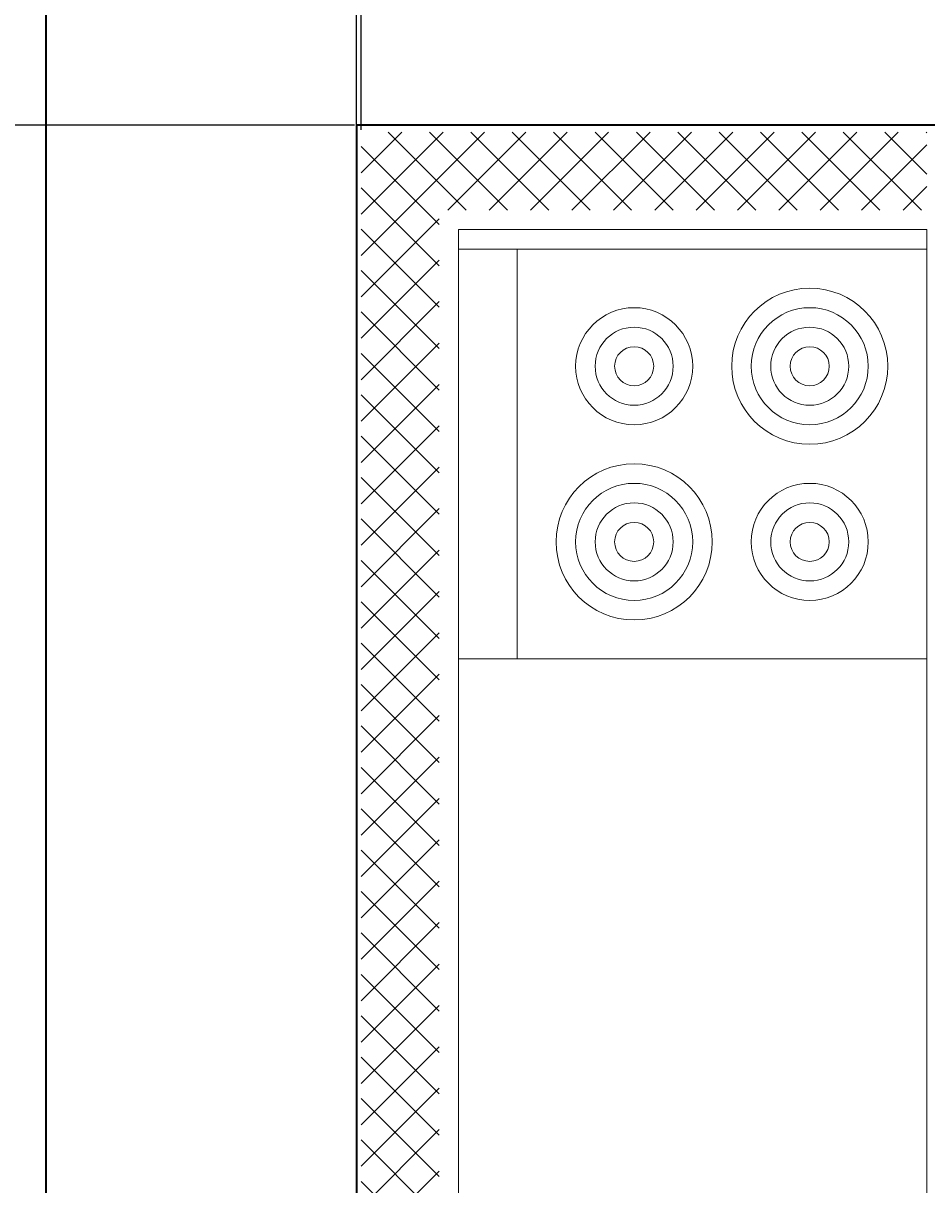
# Model space of a CAD drawing. Units: inches. Extents: x 4159 to 4826, y 299 to 1026.
# Tile 15 of 37: x 4192 to 4218, y 630 to 663. Entities that reach past the tile are written whole.
import ezdxf

# ---------------------------------------------------------------- set-up
doc = ezdxf.new("R2010")
doc.units = ezdxf.units.IN
for name, color, linetype, lineweight in [('A-ANNO-DIMS', 2, 'Continuous', 18), ('A-FLOR-FIXT', 9, 'Continuous', 18), ('A-WALL', 7, 'Continuous', 35)]:
    doc.layers.add(name, color=color, linetype=linetype, lineweight=lineweight)
doc.styles.get("Standard").update_dxf_attribs({"font": 'arial.ttf'})
doc.dimstyles.get("Standard").update_dxf_attribs({"dimtxt": 0.18, "dimasz": 0.18, "dimexe": 0.18, "dimexo": 0.0625, "dimgap": 0.09, "dimtad": 0, "dimtih": 1, "dimtoh": 1, "dimdec": 4, "dimzin": 0, "dimdsep": 46, "dimtxsty": 'Standard', "dimcen": 0.09, "dimadec": 0, "dimazin": 0, "dimtfac": 1, "dimtdec": 4, "dimtofl": 0, "dimtmove": 0, "dimatfit": 3, "dimfxl": 1, "dimtolj": 1, "dimtzin": 0, "dimarcsym": 0})

# ---------------------------------------------------------------- blocks, each defined once
blk = doc.blocks.new('Kitchen Layout - 7 x 8 ft')
for p, q in [((43.232, 85), (47.232, 89)), ((47.762, 85), (43.762, 89)), ((45.353, 85), (49.353, 89)), ((49.883, 85), (45.883, 89)), ((47.475, 85), (51.475, 89)), ((52.004, 85), (48.004, 89)), ((49.596, 85), (53.596, 89)), ((54.126, 85), (50.126, 89)), ((51.717, 85), (55.717, 89)), ((56.247, 85), (52.247, 89)), ((53.839, 85), (57.839, 89)), ((58.368, 85), (54.368, 89)), ((55.96, 85), (59.96, 89)), ((60.49, 85), (56.49, 89)), ((58.081, 85), (62.081, 89)), ((62.611, 85), (58.611, 89)), ((60.203, 85), (64.203, 89)), ((64.732, 85), (60.732, 89)), ((62.324, 85), (66.324, 89)), ((66.854, 85), (62.854, 89)), ((64.445, 85), (68.445, 89)), ((68.975, 85), (64.975, 89)), ((66.567, 85), (70.567, 89)), ((71.096, 85), (67.096, 89)), ((68.688, 85), (72.688, 89)), ((73.218, 85), (69.218, 89)), ((70.809, 85), (74.809, 89)), ((75.339, 85), (71.339, 89)), ((72.931, 85), (76.931, 89)), ((77.46, 85), (73.46, 89)), ((75.052, 85), (79.052, 89)), ((79.582, 85), (75.582, 89)), ((77.173, 85), (81.173, 89)), ((81.703, 85), (77.703, 89)), ((79.295, 85), (83.295, 89)), ((83.824, 85), (79.824, 89)), ((81.416, 85), (85.416, 89)), ((85.946, 85), (81.946, 89)), ((83.537, 85), (87.537, 89)), ((88.067, 85), (84.067, 89)), ((85.658, 85), (89.658, 89)), ((90.188, 85), (86.188, 89)), ((87.78, 85), (91.78, 89)), ((92.309, 85), (88.309, 89)), ((89.901, 85), (93.901, 89)), ((94.431, 85), (90.431, 89)), ((92.022, 85), (96.022, 89)), ((96.552, 85), (92.552, 89)), ((94.144, 85), (98.144, 89)), ((101, 82.673), (94.673, 89)), ((96.265, 85), (100.265, 89)), ((101, 84.795), (96.795, 89)), ((101, 86.916), (98.916, 89)), ((97, 83.614), (101, 87.614)), ((97, 81.492), (101, 85.492)), ((101, 80.552), (97, 84.552)), ((34, 84), (96, 84)), ((96, 84), (96, 60)), ((97, 79.371), (101, 83.371)), ((101, 78.431), (97, 82.431)), ((74, 81), (95, 81)), ((97, 77.25), (101, 81.25)), ((101, 76.309), (97, 80.309)), ((97, 75.128), (101, 79.128)), ((101, 74.188), (97, 78.188)), ((97, 73.007), (101, 77.007)), ((101, 72.067), (97, 76.067)), ((97, 70.886), (101, 74.886)), ((101, 69.946), (97, 73.946)), ((97, 68.764), (101, 72.764)), ((101, 67.824), (97, 71.824)), ((97, 66.643), (101, 70.643)), ((101, 65.703), (97, 69.703)), ((97, 64.522), (101, 68.522)), ((101, 63.582), (97, 67.582)), ((97, 62.4), (101, 66.4)), ((101, 61.46), (97, 65.46)), ((97, 60.279), (101, 64.279)), ((100.339, 60), (97, 63.339)), ((98.842, 60), (101, 62.158)), ((98.218, 60), (97, 61.218)), ((96, 60), (34, 60)), ((100.964, 60), (101, 60.036))]:
    blk.add_line(p, q)
blk.add_lwpolyline([(74, 60), (74, 84), (95, 84), (95, 60)], close=True)
for centre, radius in [((80, 75), 4), ((80, 75), 3), ((89, 75), 3), ((80, 75), 2), ((89, 75), 2), ((80, 75), 1), ((89, 75), 1), ((89, 66), 4), ((80, 66), 3), ((89, 66), 3), ((80, 66), 2), ((89, 66), 2), ((80, 66), 1), ((89, 66), 1)]:
    blk.add_circle(centre, radius)
blk = doc.blocks.new('*D40')
at = {"layer": 'A-ANNO-DIMS', "color": 0, "lineweight": -2, "transparency": 16777216}
for p, q in [((4201.437, 660.122), (4201.437, 669.224)), ((4201.617, 669.044), (4227.465, 669.044)), ((4254.37, 669.044), (4228.521, 669.044)), ((4254.55, 660.122), (4254.55, 669.224))]:
    blk.add_line(p, q, dxfattribs=at)
at = {"layer": 'A-ANNO-DIMS', "color": 0, "transparency": 16777216}
for points in [[(4201.617, 669.074), (4201.617, 669.014), (4201.437, 669.044)], [(4254.37, 669.074), (4254.37, 669.014), (4254.55, 669.044)]]:
    blk.add_solid(points, dxfattribs=at)
at = {"layer": 'Defpoints', "color": 0, "transparency": 16777216}
for p in [(4201.437, 669.044), (4201.437, 660.06), (4254.55, 660.06)]:
    blk.add_point(p, dxfattribs=at)
at = {"layer": 'A-ANNO-DIMS', "color": 0, "transparency": 16777216, "insert": (4227.993, 669.044), "char_height": 0.18, "attachment_point": 5}
blk.add_mtext('\\A1;53 TYP.', dxfattribs=at)
blk = doc.blocks.new('*D44')
at = {"layer": 'A-ANNO-DIMS', "color": 0, "lineweight": -2, "transparency": 16777216}
for p, q in [((4287.263, 963.093), (4158.88, 963.093)), ((4159.06, 962.913), (4159.06, 647.826)), ((4159.06, 332.375), (4159.06, 647.462)), ((4447.248, 332.195), (4158.88, 332.195))]:
    blk.add_line(p, q, dxfattribs=at)
at = {"layer": 'A-ANNO-DIMS', "color": 0, "transparency": 16777216}
for points in [[(4159.03, 962.913), (4159.09, 962.913), (4159.06, 963.093)], [(4159.03, 332.375), (4159.09, 332.375), (4159.06, 332.195)]]:
    blk.add_solid(points, dxfattribs=at)
at = {"layer": 'Defpoints', "color": 0, "transparency": 16777216}
for p in [(4287.326, 963.093), (4159.06, 332.195), (4447.31, 332.195)]:
    blk.add_point(p, dxfattribs=at)
at = {"layer": 'A-ANNO-DIMS', "color": 0, "transparency": 16777216, "insert": (4159.06, 647.644), "char_height": 0.18, "attachment_point": 5}
blk.add_mtext('\\A1;630.9', dxfattribs=at)
blk = doc.blocks.new('*D50')
at = {"layer": 'A-ANNO-DIMS', "color": 0, "lineweight": -2, "transparency": 16777216}
for p, q in [((4192.31, 392.317), (4192.31, 1025.842)), ((4201.31, 401.317), (4201.31, 1025.842)), ((4192.49, 1025.662), (4196.661, 1025.662)), ((4201.13, 1025.662), (4196.959, 1025.662))]:
    blk.add_line(p, q, dxfattribs=at)
at = {"layer": 'A-ANNO-DIMS', "color": 0, "transparency": 16777216}
for points in [[(4192.49, 1025.692), (4192.49, 1025.632), (4192.31, 1025.662)], [(4201.13, 1025.692), (4201.13, 1025.632), (4201.31, 1025.662)]]:
    blk.add_solid(points, dxfattribs=at)
at = {"layer": 'Defpoints', "color": 0, "transparency": 16777216}
for p in [(4201.31, 1025.662), (4201.31, 401.254), (4192.31, 392.254)]:
    blk.add_point(p, dxfattribs=at)
at = {"layer": 'A-ANNO-DIMS', "color": 0, "transparency": 16777216, "insert": (4196.81, 1025.662), "char_height": 0.18, "attachment_point": 5}
blk.add_mtext('\\A1;9', dxfattribs=at)
blk = doc.blocks.new('*D51')
at = {"layer": 'A-ANNO-DIMS', "color": 0, "lineweight": -2, "transparency": 16777216}
for p, q in [((4201.248, 660.254), (4158.88, 660.254)), ((4159.06, 660.074), (4159.06, 526.436)), ((4159.06, 392.434), (4159.06, 526.072)), ((4192.248, 392.254), (4158.88, 392.254))]:
    blk.add_line(p, q, dxfattribs=at)
at = {"layer": 'A-ANNO-DIMS', "color": 0, "transparency": 16777216}
for points in [[(4159.03, 660.074), (4159.09, 660.074), (4159.06, 660.254)], [(4159.03, 392.434), (4159.09, 392.434), (4159.06, 392.254)]]:
    blk.add_solid(points, dxfattribs=at)
at = {"layer": 'Defpoints', "color": 0, "transparency": 16777216}
for p in [(4159.06, 660.254), (4201.31, 660.254), (4192.31, 392.254)]:
    blk.add_point(p, dxfattribs=at)
at = {"layer": 'A-ANNO-DIMS', "color": 0, "transparency": 16777216, "insert": (4159.06, 526.254), "char_height": 0.18, "attachment_point": 5}
blk.add_mtext('\\A1;268', dxfattribs=at)

msp = doc.modelspace()

# ---------------------------------------------------------------- linework, layer by layer
at = {"layer": 'A-WALL'}
for p, q in [((4447.31, 660.254), (4201.31, 660.254)), ((4201.31, 660.254), (4201.31, 600.254))]:
    msp.add_line(p, q, dxfattribs=at)
msp.add_lwpolyline([(4303.31, 903.254), (4192.31, 903.254), (4192.31, 392.254)], dxfattribs=at)

# ---------------------------------------------------------------- block references
at = {"layer": 'A-FLOR-FIXT', "xscale": 0.5650329326971529, "yscale": 0.5650329326971529, "zscale": 0.5650329326971529, "rotation": 90}
msp.add_blockref('Kitchen Layout - 7 x 8 ft', (4251.725, 602.991), dxfattribs=at)

# ---------------------------------------------------------------- dimensions: what is measured, and where the dimension line sits
at = {"layer": 'A-ANNO-DIMS'}
dim = msp.add_linear_dim(base=(4201.31, 1025.662), p1=(4192.31, 392.254), p2=(4201.31, 401.254), dimstyle='Standard', override={"dimdec": 0, "dimlfac": 1, "dimrnd": 0, "dimzin": 0, "dimdsep": 46, "dimlunit": 2}, dxfattribs=at)
dim.commit()
dim.dimension.update_dxf_attribs({"geometry": '*D50', "text_midpoint": (4196.81, 1025.662)})
for base, p1, p2, override, picture, middle in [((4159.06, 332.195), (4287.326, 963.093), (4447.31, 332.195), {"dimdec": 1, "dimlfac": 1, "dimrnd": 0, "dimzin": 0, "dimdsep": 46, "dimlunit": 2}, '*D44', (4159.06, 647.644)), ((4159.06, 660.254), (4192.31, 392.254), (4201.31, 660.254), {"dimdec": 0, "dimlfac": 1, "dimrnd": 0, "dimzin": 0, "dimdsep": 46, "dimlunit": 2}, '*D51', (4159.06, 526.254))]:
    dim = msp.add_linear_dim(base=base, p1=p1, p2=p2, angle=90, dimstyle='Standard', override=override, dxfattribs=at)
    dim.commit()
    dim.dimension.update_dxf_attribs({"geometry": picture, "text_midpoint": middle})
dim = msp.add_linear_dim(base=(4201.437, 669.044), p1=(4254.55, 660.06), p2=(4201.437, 660.06), angle=180, text='<> TYP.', dimstyle='Standard', override={"dimdec": 0, "dimlfac": 1, "dimrnd": 0, "dimzin": 0, "dimdsep": 46, "dimlunit": 2}, dxfattribs=at)
dim.commit()
dim.dimension.update_dxf_attribs({"geometry": '*D40', "text_midpoint": (4227.993, 669.044)})

doc.saveas('drawing.dxf')
